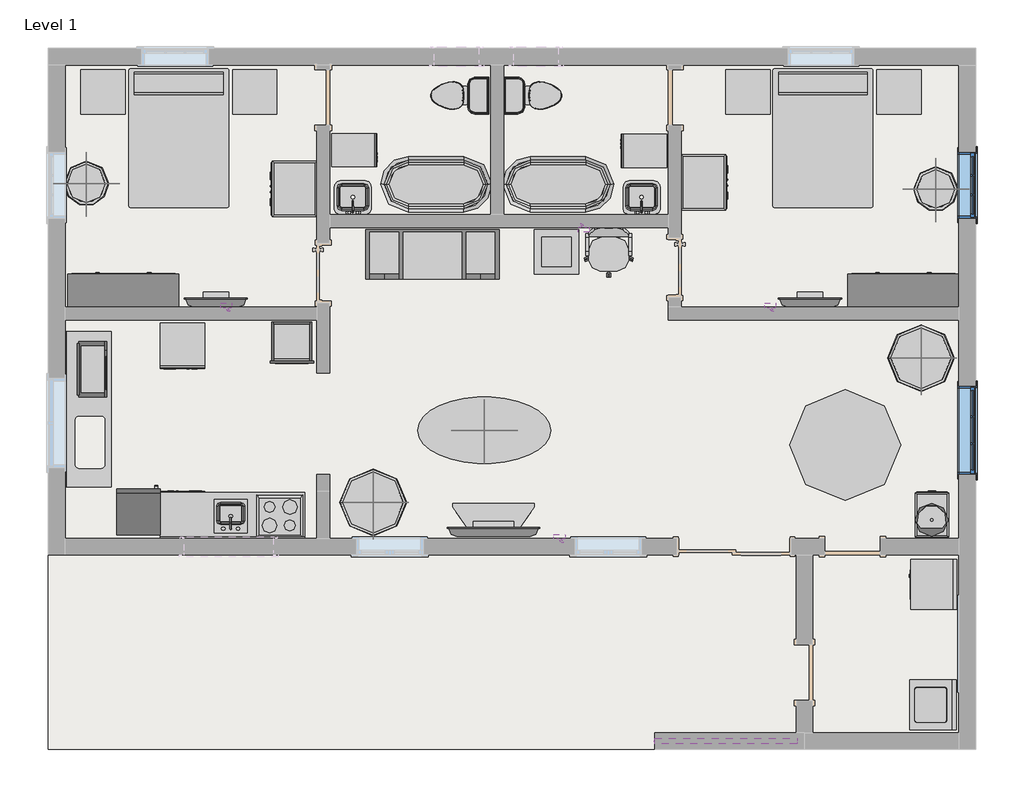
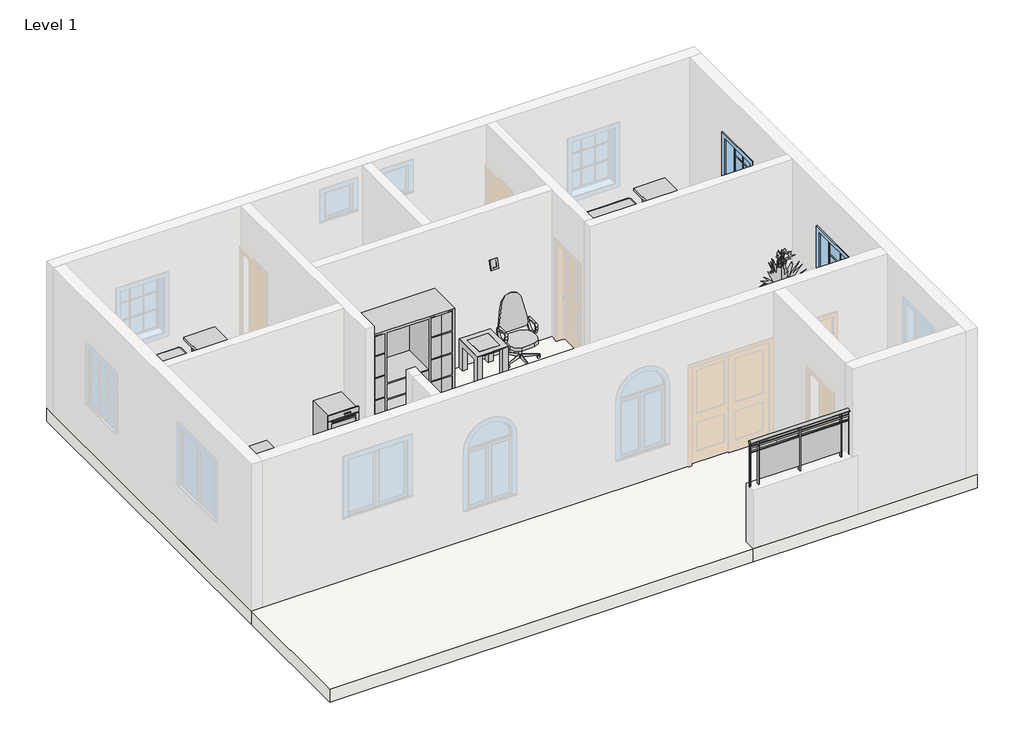
# One storey, part 2 of 2: 26 furniture elements, 15 proxies, 11 flow terminals, 5 geographic elements, 2 windows, 1 railing, 1 slab.
"""IFC4 building model written with IfcOpenShell, lengths in millimetres."""

from ifc_helpers import new_model, si_unit, point, frame, origin, place, context, project, spatial, polyline, ellipse_curve, trimmed, outline, extrude, transform, mapped, element, save
from ifc_brep_helpers import plane_surface, extruded_surface, advanced_brep
from components import proxy_7e1014cc, proxy_a6faaae8, proxy_45b28599, proxy_b4d0e45e, kitchenette_medium_kitchenette_medium_844211aa, proxy_8a8d5ab2, proxy_8b8c2dc4, rpc_picture_frame_rpc_picture_frame_c25e3fe9, proxy_c523a7b7, proxy_718fa39f, flow_terminal_accce45a, flow_terminal_871c2e40, flow_terminal_d49f872f, flow_terminal_62a433f7, toilet_domestic_3d_toilet_domestic_3d_f7549cf7, toilet_domestic_3d_toilet_domestic_3d_183bbd19, flow_terminal_b374fae2, furniture_338da5bd, furniture_fb2da572, furniture_0253826f, chair_executive_chair_executive_8d69e98c, furniture_c6510c7c, furniture_ac03d711, furniture_06d35bcb, furniture_cf0b6580, furniture_56245f3a, furniture_fdf74506, tv_stand_tv_stand_6ce107e5, furniture_b5c51a22, furniture_bbcc68ce, furniture_027a2ad9, furniture_5bc9ed15, table_round_2_c80d6d9c, furniture_a0cc3393, rpc_plant_tropical_55f6ff97, rpc_plant_tropical_agave_1_5_93a2a214, window_642cfea4, window_544f1267

model = new_model("IFC4")

# Units and contexts
model_context = context("Model", 3, world=origin())
ifc_project = project(units=[si_unit("LENGTHUNIT", "METRE", prefix="MILLI")], contexts=[model_context])

# Site, building, storey
site = spatial("IfcSite", under=ifc_project)
building = spatial("IfcBuilding", under=site)
storey = spatial("IfcBuildingStorey", under=building, Name="Level 1", Elevation=0.0)

# Proxies
placement = place(None, origin())
proxy_shape = proxy_7e1014cc(model_context)
element("IfcBuildingElementProxy", 1, Name="18\" x 24\" x 34 1/2\"", ObjectType="18\" x 24\" x 34 1/2\"", at=placement, inside=storey, context=model_context, shape_type="MappedRepresentation", body=[
    mapped(proxy_shape, transform((-2868.9943199, 12467.072386, 0.0), x_axis=(0.0, -1.0000000000000004, 0.0), y_axis=(1.0000000000000004, 0.0, 0.0), z_axis=(0.0, 0.0, 1.0))),
])
element("IfcBuildingElementProxy", 2, Name="18\" x 24\" x 34 1/2\"", ObjectType="18\" x 24\" x 34 1/2\"", at=placement, inside=storey, context=model_context, shape_type="MappedRepresentation", body=[
    mapped(proxy_shape, transform((-6323.8951903, 11867.537449, 0.0), x_axis=(0.0, 1.0, 0.0), y_axis=(-1.0, 0.0, 0.0), z_axis=(0.0, 0.0, 1.0))),
])
proxy_2_shape = proxy_a6faaae8(model_context)
element("IfcBuildingElementProxy", 3, Name="Cook Top-4 Unit2 : 22\" x 20\"", ObjectType="Cook Top-4 Unit2 : 22\" x 20\"", at=placement, inside=storey, context=model_context, shape_type="MappedRepresentation", body=[
    mapped(proxy_2_shape, transform((-7606.3447551, 7144.4549175, 0.0), x_axis=(-1.0000000000000004, 0.0, 0.0), y_axis=(0.0, -1.0000000000000004, 0.0), z_axis=(0.0, 0.0, 1.0))),
])
proxy_3_shape = proxy_45b28599(model_context)
element("IfcBuildingElementProxy", 4, Name="Dishwasher : 24\" x 24\" x 34\"", ObjectType="Dishwasher : 24\" x 24\" x 34\"", at=placement, inside=storey, context=model_context, shape_type="MappedRepresentation", body=[
    mapped(proxy_3_shape, transform((-8557.5272866, 7436.3044823, 0.0), x_axis=(-1.0000000000000004, 0.0, 0.0), y_axis=(0.0, -1.0000000000000004, 0.0), z_axis=(0.0, 0.0, 1.0))),
])
element("IfcBuildingElementProxy", 5, Name="Dishwasher : 24\" x 24\" x 34\"", ObjectType="Dishwasher : 24\" x 24\" x 34\"", at=placement, inside=storey, context=model_context, shape_type="MappedRepresentation", body=[
    mapped(proxy_3_shape, transform((-9322.1622236, 9227.5053528, 0.0), x_axis=(1.0, 0.0, 0.0), y_axis=(0.0, 1.0, 0.0), z_axis=(0.0, 0.0, 1.0))),
])
proxy_4_shape = proxy_b4d0e45e(model_context)
element("IfcBuildingElementProxy", 6, Name="Dryer : 27\" x 25\" x 35\"", ObjectType="Dryer : 27\" x 25\" x 35\"", at=placement, inside=storey, context=model_context, shape_type="MappedRepresentation", body=[
    mapped(proxy_4_shape, transform((1055.0552449, 6585.6549175, 0.0), x_axis=(0.0, -1.0000000000000004, 0.0), y_axis=(1.0000000000000004, 0.0, 0.0), z_axis=(0.0, 0.0, 1.0))),
])
kitchenette_medium_kitchenette_medium_shape = kitchenette_medium_kitchenette_medium_844211aa(model_context)
element("IfcBuildingElementProxy", 7, Name="Kitchenette - Medium : Kitchenette - Medium", ObjectType="Kitchenette - Medium : Kitchenette - Medium", at=placement, inside=storey, context=model_context, shape_type="MappedRepresentation", body=[
    mapped(kitchenette_medium_kitchenette_medium_shape, transform((-7930.5070502, 6839.6549175, 0.0), x_axis=(-1.0000000000000004, 0.0, 0.0), y_axis=(0.0, -1.0000000000000004, 0.0), z_axis=(0.0, 0.0, 1.0))),
])
proxy_5_shape = proxy_8a8d5ab2(model_context)
element("IfcBuildingElementProxy", 8, Name="Microwave : 30\" x 16\" x 18\"", ObjectType="Microwave : 30\" x 16\" x 18\"", at=placement, inside=storey, context=model_context, shape_type="MappedRepresentation", body=[
    mapped(proxy_5_shape, transform((-10537.525261, 8663.4620402, 0.0), x_axis=(0.0, 1.0, 0.0), y_axis=(-1.0, 0.0, 0.0), z_axis=(0.0, 0.0, 1.0))),
])
proxy_6_shape = proxy_8b8c2dc4(model_context)
element("IfcBuildingElementProxy", 9, Name="Oven Double-Built-in : 21 1/2\" x 39 1/4\" x 21\"", ObjectType="Oven Double-Built-in : 21 1/2\" x 39 1/4\" x 21\"", at=placement, inside=storey, context=model_context, shape_type="MappedRepresentation", body=[
    mapped(proxy_6_shape, transform((-7406.0698278, 9403.6890586, 0.0), x_axis=(1.0, 0.0, 0.0), y_axis=(0.0, 1.0, 0.0), z_axis=(0.0, 0.0, 1.0))),
])
rpc_picture_frame_rpc_picture_frame_shape = rpc_picture_frame_rpc_picture_frame_c25e3fe9(model_context)
element("IfcBuildingElementProxy", 10, Name="RPC Picture Frame : RPC Picture Frame", ObjectType="RPC Picture Frame : RPC Picture Frame", at=placement, inside=storey, context=model_context, shape_type="MappedRepresentation", body=[
    mapped(rpc_picture_frame_rpc_picture_frame_shape, transform((-8339.9401773, 10014.6549175, 1828.8), x_axis=(-1.0000000000000004, 0.0, 0.0), y_axis=(0.0, -1.0000000000000004, 0.0), z_axis=(0.0, 0.0, 1.0))),
])
element("IfcBuildingElementProxy", 11, Name="RPC Picture Frame : RPC Picture Frame", ObjectType="RPC Picture Frame : RPC Picture Frame", at=placement, inside=storey, context=model_context, shape_type="MappedRepresentation", body=[
    mapped(rpc_picture_frame_rpc_picture_frame_shape, transform((-876.145624, 10014.6549175, 1828.8), x_axis=(-1.0, 0.0, 0.0), y_axis=(0.0, -1.0, 0.0), z_axis=(0.0, 0.0, 1.0))),
])
element("IfcBuildingElementProxy", 12, Name="RPC Picture Frame : RPC Picture Frame", ObjectType="RPC Picture Frame : RPC Picture Frame", at=placement, inside=storey, context=model_context, shape_type="MappedRepresentation", body=[
    mapped(rpc_picture_frame_rpc_picture_frame_shape, transform((-3766.7525994, 6839.6549175, 1828.8), x_axis=(-1.0000000000000004, 0.0, 0.0), y_axis=(0.0, -1.0000000000000004, 0.0), z_axis=(0.0, 0.0, 1.0))),
])
element("IfcBuildingElementProxy", 13, Name="RPC Picture Frame : RPC Picture Frame", ObjectType="RPC Picture Frame : RPC Picture Frame", at=placement, inside=storey, context=model_context, shape_type="MappedRepresentation", body=[
    mapped(rpc_picture_frame_rpc_picture_frame_shape, transform((-3433.7801384, 11106.8549175, 1828.8), x_axis=(1.0, 0.0, 0.0), y_axis=(0.0, 1.0, 0.0), z_axis=(0.0, 0.0, 1.0))),
])
proxy_7_shape = proxy_c523a7b7(model_context)
element("IfcBuildingElementProxy", 14, Name="Refrigerator : 24\" x 25\" LH", ObjectType="Refrigerator : 24\" x 25\" LH", at=placement, inside=storey, context=model_context, shape_type="MappedRepresentation", body=[
    mapped(proxy_7_shape, transform((-9543.0947551, 7190.103889, 0.0), x_axis=(-1.0000000000000004, 0.0, 0.0), y_axis=(0.0, -1.0000000000000004, 0.0), z_axis=(0.0, 0.0, 1.0))),
])
proxy_8_shape = proxy_718fa39f(model_context)
element("IfcBuildingElementProxy", 15, Name="Washer : 27\" x 25\" x 35\"", ObjectType="Washer : 27\" x 25\" x 35\"", at=placement, inside=storey, context=model_context, shape_type="MappedRepresentation", body=[
    mapped(proxy_8_shape, transform((1080.7056801, 4974.072386, 0.0), x_axis=(0.0, -1.0, 0.0), y_axis=(1.0, 0.0, 0.0), z_axis=(0.0, 0.0, 1.0))),
])

# Flow terminals
flow_terminal_shape = flow_terminal_accce45a(model_context)
element("IfcFlowTerminal", 16, ObjectType="Floor Drain - Round : 5\" Strainer - 2\" Drain", at=placement, inside=storey, context=model_context, shape_type="MappedRepresentation", body=[
    mapped(flow_terminal_shape, transform((-4291.6447551, 12313.3549175, 0.0), x_axis=(1.0, 0.0, 0.0), y_axis=(0.0, 1.0, 0.0), z_axis=(0.0, 0.0, 1.0))),
])
element("IfcFlowTerminal", 17, ObjectType="Floor Drain - Round : 5\" Strainer - 2\" Drain", at=placement, inside=storey, context=model_context, shape_type="MappedRepresentation", body=[
    mapped(flow_terminal_shape, transform((-4952.0447551, 12338.7549175, 0.0), x_axis=(1.0, 0.0, 0.0), y_axis=(0.0, 1.0, 0.0), z_axis=(0.0, 0.0, 1.0))),
])
element("IfcFlowTerminal", 18, ObjectType="Floor Drain - Round : 5\" Strainer - 2\" Drain", at=placement, inside=storey, context=model_context, shape_type="MappedRepresentation", body=[
    mapped(flow_terminal_shape, transform((788.3552449, 4337.7549175, 0.0), x_axis=(0.0, 1.0, 0.0), y_axis=(-1.0, 0.0, 0.0), z_axis=(0.0, 0.0, 1.0))),
])
flow_terminal_2_shape = flow_terminal_871c2e40(model_context)
element("IfcFlowTerminal", 19, ObjectType="Sink Kitchen-Island : 18\" x 18\"", at=placement, inside=storey, context=model_context, shape_type="MappedRepresentation", body=[
    mapped(flow_terminal_2_shape, transform((-8263.7555146, 7146.8003187, -14.4), x_axis=(-1.0000000000000004, 0.0, 0.0), y_axis=(0.0, -1.0000000000000004, 0.0), z_axis=(0.0, 0.0, 1.0))),
])
flow_terminal_3_shape = flow_terminal_d49f872f(model_context)
element("IfcFlowTerminal", 20, ObjectType="Sink Vanity-Round : 19\" x 19\"", at=placement, inside=storey, context=model_context, shape_type="MappedRepresentation", body=[
    mapped(flow_terminal_3_shape, transform((1437.4569854, 7180.500516, 431.8), x_axis=(-1.0000000000000004, 0.0, 0.0), y_axis=(0.0, -1.0000000000000004, 0.0), z_axis=(0.0, 0.0, 1.0))),
])
flow_terminal_4_shape = flow_terminal_62a433f7(model_context)
element("IfcFlowTerminal", 21, ObjectType="Sink Vanity-Square : 20\" x 18\"", at=placement, inside=storey, context=model_context, shape_type="MappedRepresentation", body=[
    mapped(flow_terminal_4_shape, transform((-6587.3555146, 11477.5003187, 0.0), x_axis=(-1.0000000000000004, 0.0, 0.0), y_axis=(0.0, -1.0000000000000004, 0.0), z_axis=(0.0, 0.0, 1.0))),
])
element("IfcFlowTerminal", 22, ObjectType="Sink Vanity-Square : 20\" x 18\"", at=placement, inside=storey, context=model_context, shape_type="MappedRepresentation", body=[
    mapped(flow_terminal_4_shape, transform((-2624.9555146, 11477.5003187, 0.0), x_axis=(-1.0, 0.0, 0.0), y_axis=(0.0, -1.0, 0.0), z_axis=(0.0, 0.0, 1.0))),
])
toilet_domestic_3d_toilet_domestic_3d_shape = toilet_domestic_3d_toilet_domestic_3d_f7549cf7(model_context)
toilet_domestic_3d_toilet_domestic_3d_2_shape = toilet_domestic_3d_toilet_domestic_3d_183bbd19(model_context)
element("IfcFlowTerminal", 23, ObjectType="Toilet-Domestic-3D : Toilet-Domestic-3D", at=placement, inside=storey, context=model_context, shape_type="MappedRepresentation", body=[
    mapped(toilet_domestic_3d_toilet_domestic_3d_shape, transform((-5230.8407825, 12922.9549175, 0.0), x_axis=(0.0, -1.0000000000000004, 0.0), y_axis=(1.0000000000000004, 0.0, 0.0), z_axis=(0.0, 0.0, 1.0))),
    mapped(toilet_domestic_3d_toilet_domestic_3d_2_shape, transform((-5230.8407825, 12922.9549175, 0.0), x_axis=(0.0, -1.0000000000000004, 0.0), y_axis=(1.0000000000000004, 0.0, 0.0), z_axis=(0.0, 0.0, 1.0))),
])
element("IfcFlowTerminal", 24, ObjectType="Toilet-Domestic-3D : Toilet-Domestic-3D", at=placement, inside=storey, context=model_context, shape_type="MappedRepresentation", body=[
    mapped(toilet_domestic_3d_toilet_domestic_3d_shape, transform((-4038.2487278, 12922.9549175, 0.0), x_axis=(0.0, 1.0000000000000004, 0.0), y_axis=(-1.0000000000000004, 0.0, 0.0), z_axis=(0.0, 0.0, 1.0))),
    mapped(toilet_domestic_3d_toilet_domestic_3d_2_shape, transform((-4038.2487278, 12922.9549175, 0.0), x_axis=(0.0, 1.0000000000000004, 0.0), y_axis=(-1.0000000000000004, 0.0, 0.0), z_axis=(0.0, 0.0, 1.0))),
])
flow_terminal_5_shape = flow_terminal_b374fae2(model_context)
element("IfcFlowTerminal", 25, ObjectType="Tub-Free Standing-3D : 30\" x 60\"", at=placement, inside=storey, context=model_context, shape_type="MappedRepresentation", body=[
    mapped(flow_terminal_5_shape, transform((-5460.0447551, 11703.7549175, 0.0), x_axis=(0.0, -1.0000000000000004, 0.0), y_axis=(1.0000000000000004, 0.0, 0.0), z_axis=(0.0, 0.0, 1.0))),
])
element("IfcFlowTerminal", 26, ObjectType="Tub-Free Standing-3D : 30\" x 60\"", at=placement, inside=storey, context=model_context, shape_type="MappedRepresentation", body=[
    mapped(flow_terminal_5_shape, transform((-3784.2487278, 11703.7549175, 0.0), x_axis=(0.0, 1.0000000000000002, 0.0), y_axis=(-1.0000000000000002, 0.0, 0.0), z_axis=(0.0, 0.0, 1.0))),
])

# Furniture
furniture_shape = furniture_338da5bd(model_context)
element("IfcFurniture", 27, ObjectType="30\"", at=placement, inside=storey, context=model_context, shape_type="MappedRepresentation", body=[
    mapped(furniture_shape, transform((-2094.5447551, 11710.4172126, 0.0), x_axis=(0.0, 1.0000000000000002, 0.0), y_axis=(-1.0000000000000002, 0.0, 0.0), z_axis=(0.0, 0.0, 1.0))),
])
element("IfcFurniture", 28, ObjectType="30\"", at=placement, inside=storey, context=model_context, shape_type="MappedRepresentation", body=[
    mapped(furniture_shape, transform((-7098.3447551, 11658.9926225, 0.0), x_axis=(0.0, -1.0000000000000002, 0.0), y_axis=(1.0000000000000002, 0.0, 0.0), z_axis=(0.0, 0.0, 1.0))),
])
furniture_2_shape = furniture_fb2da572(model_context)
element("IfcFurniture", 29, ObjectType="Base Cabinet-4 Drawers : 18\"", at=placement, inside=storey, context=model_context, shape_type="MappedRepresentation", body=[
    mapped(furniture_2_shape, transform((1365.8929498, 6858.7049175, 0.0), x_axis=(-1.0, 0.0, 0.0), y_axis=(0.0, -1.0, 0.0), z_axis=(0.0, 0.0, 1.0))),
])
furniture_3_shape = furniture_0253826f(model_context)
element("IfcFurniture", 30, ObjectType="Bed-Standard.0001 : Double 54\" x 75\"", at=placement, inside=storey, context=model_context, shape_type="MappedRepresentation", body=[
    mapped(furniture_3_shape, transform((-9262.1332797, 12384.3499995, 0.0), x_axis=(1.0, 0.0, 0.0), y_axis=(0.0, 1.0, 0.0), z_axis=(0.0, 0.0, 1.0))),
])
element("IfcFurniture", 31, ObjectType="Bed-Standard.0001 : Double 54\" x 75\"", at=placement, inside=storey, context=model_context, shape_type="MappedRepresentation", body=[
    mapped(furniture_3_shape, transform((-422.9332797, 12384.3499995, 0.0), x_axis=(1.0, 0.0, 0.0), y_axis=(0.0, 1.0, 0.0), z_axis=(0.0, 0.0, 1.0))),
])
chair_executive_chair_executive_shape = chair_executive_chair_executive_8d69e98c(model_context)
element("IfcFurniture", 32, ObjectType="Chair-Executive : Chair-Executive", at=placement, inside=storey, context=model_context, shape_type="MappedRepresentation", body=[
    mapped(chair_executive_chair_executive_shape, transform((-2950.5039355, 10795.6008192, 0.0), x_axis=(-1.0000000000000004, 0.0, 0.0), y_axis=(0.0, -1.0000000000000004, 0.0), z_axis=(0.0, 0.0, 1.0))),
])
furniture_4_shape = furniture_c6510c7c(model_context)
element("IfcFurniture", 33, ObjectType="Counter Top w Sink Hole : 24\" Depth", at=placement, inside=storey, context=model_context, shape_type="MappedRepresentation", body=[
    mapped(furniture_4_shape, transform((-8463.9070502, 6839.6549175, -14.4), x_axis=(-1.0000000000000004, 0.0, 0.0), y_axis=(0.0, -1.0000000000000004, 0.0), z_axis=(0.0, 0.0, 1.0))),
])
furniture_5_shape = furniture_ac03d711(model_context)
element("IfcFurniture", 34, ObjectType="Counter Top w Sink Hole : 24\" Depth", at=placement, inside=storey, context=model_context, shape_type="MappedRepresentation", body=[
    mapped(furniture_5_shape, transform((-10552.7447551, 8751.3172126, 0.0), x_axis=(0.0, 1.0000000000000002, 0.0), y_axis=(-1.0000000000000002, 0.0, 0.0), z_axis=(0.0, 0.0, 1.0))),
])
furniture_6_shape = furniture_06d35bcb(model_context)
element("IfcFurniture", 35, ObjectType="Dresser : 72\" x 60\" x 18\"", at=placement, inside=storey, context=model_context, shape_type="MappedRepresentation", body=[
    mapped(furniture_6_shape, transform((-10021.838015, 9880.0919634, 0.0), x_axis=(-1.0000000000000004, 0.0, 0.0), y_axis=(0.0, -1.0000000000000004, 0.0), z_axis=(0.0, 0.0, 1.0))),
])
element("IfcFurniture", 36, ObjectType="Dresser : 72\" x 60\" x 18\"", at=placement, inside=storey, context=model_context, shape_type="MappedRepresentation", body=[
    mapped(furniture_6_shape, transform((684.261985, 9880.0919634, 0.0), x_axis=(-1.0000000000000004, 0.0, 0.0), y_axis=(0.0, -1.0000000000000004, 0.0), z_axis=(0.0, 0.0, 1.0))),
])
furniture_7_shape = furniture_cf0b6580(model_context)
element("IfcFurniture", 37, ObjectType="Entertainment Center : 72\" x 72\" x 24\"", at=placement, inside=storey, context=model_context, shape_type="MappedRepresentation", body=[
    mapped(furniture_7_shape, transform((-5510.8447551, 11183.0549175, 0.0), x_axis=(1.0, 0.0, 0.0), y_axis=(0.0, 1.0, 0.0), z_axis=(0.0, 0.0, 1.0))),
])
furniture_8_shape = furniture_56245f3a(model_context)
element("IfcFurniture", 38, ObjectType="TV - Flat Screen : 32\"", at=placement, inside=storey, context=model_context, shape_type="MappedRepresentation", body=[
    mapped(furniture_8_shape, transform((-333.1892693, 10073.1935412, 914.4), x_axis=(-1.0, 0.0, 0.0), y_axis=(0.0, -1.0, 0.0), z_axis=(0.0, 0.0, 1.0))),
])
element("IfcFurniture", 39, ObjectType="TV - Flat Screen : 32\"", at=placement, inside=storey, context=model_context, shape_type="MappedRepresentation", body=[
    mapped(furniture_8_shape, transform((-8486.5892693, 10073.1935412, 914.4), x_axis=(-1.0000000000000004, 0.0, 0.0), y_axis=(0.0, -1.0000000000000004, 0.0), z_axis=(0.0, 0.0, 1.0))),
])
furniture_9_shape = furniture_fdf74506(model_context)
element("IfcFurniture", 40, ObjectType="TV - Flat Screen : 50\"", at=placement, inside=storey, context=model_context, shape_type="MappedRepresentation", body=[
    mapped(furniture_9_shape, transform((-4676.5892693, 6923.5935412, 914.4), x_axis=(-1.0, 0.0, 0.0), y_axis=(0.0, -1.0, 0.0), z_axis=(0.0, 0.0, 1.0))),
])
tv_stand_tv_stand_shape = tv_stand_tv_stand_6ce107e5(model_context)
element("IfcFurniture", 41, ObjectType="TV Stand : TV Stand", at=placement, inside=storey, context=model_context, shape_type="MappedRepresentation", body=[
    mapped(tv_stand_tv_stand_shape, transform((-4547.4567531, 6865.0549175, 0.0), x_axis=(-1.0000000000000004, 0.0, 0.0), y_axis=(0.0, -1.0000000000000004, 0.0), z_axis=(0.0, 0.0, 1.0))),
])
furniture_10_shape = furniture_b5c51a22(model_context)
element("IfcFurniture", 42, ObjectType="Table-Coffee : 24\" x 24\" x 24\"", at=placement, inside=storey, context=model_context, shape_type="MappedRepresentation", body=[
    mapped(furniture_10_shape, transform((-3827.3105218, 10681.4438397, 0.0), x_axis=(1.0, 0.0, 0.0), y_axis=(0.0, 1.0, 0.0), z_axis=(0.0, 0.0, 1.0))),
])
furniture_11_shape = furniture_bbcc68ce(model_context)
element("IfcFurniture", 43, ObjectType="Table-Dining Round w Chairs : 60\" Diameter", at=placement, inside=storey, context=model_context, shape_type="MappedRepresentation", body=[
    mapped(furniture_11_shape, transform((49.6732777, 8307.2336061, 0.0), x_axis=(1.0, 0.0, 0.0), y_axis=(0.0, 1.0, 0.0), z_axis=(0.0, 0.0, 1.0))),
])
furniture_12_shape = furniture_027a2ad9(model_context)
element("IfcFurniture", 44, ObjectType="Table-Ellipse : 72\" x 36\"", at=placement, inside=storey, context=model_context, shape_type="MappedRepresentation", body=[
    mapped(furniture_12_shape, transform((-4799.6447551, 8325.5549175, 0.0), x_axis=(1.0, 0.0, 0.0), y_axis=(0.0, 1.0, 0.0), z_axis=(0.0, 0.0, 1.0))),
])
furniture_13_shape = furniture_5bc9ed15(model_context)
element("IfcFurniture", 45, ObjectType="Table-Night Stand : 24\" x 24\" x 30\"", at=placement, inside=storey, context=model_context, shape_type="MappedRepresentation", body=[
    mapped(furniture_13_shape, transform((-10340.5783854, 12668.9549175, 0.0), x_axis=(1.0, 0.0, 0.0), y_axis=(0.0, 1.0, 0.0), z_axis=(0.0, 0.0, 1.0))),
])
element("IfcFurniture", 46, ObjectType="Table-Night Stand : 24\" x 24\" x 30\"", at=placement, inside=storey, context=model_context, shape_type="MappedRepresentation", body=[
    mapped(furniture_13_shape, transform((-8257.7783854, 12668.9549175, 0.0), x_axis=(1.0, 0.0, 0.0), y_axis=(0.0, 1.0, 0.0), z_axis=(0.0, 0.0, 1.0))),
])
element("IfcFurniture", 47, ObjectType="Table-Night Stand : 24\" x 24\" x 30\"", at=placement, inside=storey, context=model_context, shape_type="MappedRepresentation", body=[
    mapped(furniture_13_shape, transform((-1488.6783854, 12668.9549175, 0.0), x_axis=(1.0, 0.0, 0.0), y_axis=(0.0, 1.0, 0.0), z_axis=(0.0, 0.0, 1.0))),
])
element("IfcFurniture", 48, ObjectType="Table-Night Stand : 24\" x 24\" x 30\"", at=placement, inside=storey, context=model_context, shape_type="MappedRepresentation", body=[
    mapped(furniture_13_shape, transform((581.4216146, 12668.9549175, 0.0), x_axis=(1.0, 0.0, 0.0), y_axis=(0.0, 1.0, 0.0), z_axis=(0.0, 0.0, 1.0))),
])
table_round_2_shape = table_round_2_c80d6d9c(model_context)
element("IfcFurniture", 49, ObjectType="Table-Round : 2", at=placement, inside=storey, context=model_context, shape_type="MappedRepresentation", body=[
    mapped(table_round_2_shape, transform((1194.7552449, 9316.1549175, 0.0), x_axis=(1.0, 0.0, 0.0), y_axis=(0.0, 1.0, 0.0), z_axis=(0.0, 0.0, 1.0))),
])
element("IfcFurniture", 50, ObjectType="Table-Round : 2", at=placement, inside=storey, context=model_context, shape_type="MappedRepresentation", body=[
    mapped(table_round_2_shape, transform((-6323.6447551, 7334.9549175, 0.0), x_axis=(1.0, 0.0, 0.0), y_axis=(0.0, 1.0, 0.0), z_axis=(0.0, 0.0, 1.0))),
])
furniture_14_shape = furniture_a0cc3393(model_context)
element("IfcFurniture", 51, ObjectType="Table-Round : 36\" Diameter", at=placement, inside=storey, context=model_context, shape_type="MappedRepresentation", body=[
    mapped(furniture_14_shape, transform((1397.9552449, 11640.2549175, 0.0), x_axis=(1.0, 0.0, 0.0), y_axis=(0.0, 1.0, 0.0), z_axis=(0.0, 0.0, 1.0))),
])
element("IfcFurniture", 52, ObjectType="Table-Round : 36\" Diameter", at=placement, inside=storey, context=model_context, shape_type="MappedRepresentation", body=[
    mapped(furniture_14_shape, transform((-10260.6447551, 11716.4549175, 0.0), x_axis=(1.0, 0.0, 0.0), y_axis=(0.0, 1.0, 0.0), z_axis=(0.0, 0.0, 1.0))),
])

# Geographic elements
rpc_plant_tropical_shape = rpc_plant_tropical_55f6ff97(model_context)
element("IfcGeographicElement", 53, ObjectType="RPC Plant - Tropical", at=placement, inside=storey, context=model_context, shape_type="MappedRepresentation", body=[
    mapped(rpc_plant_tropical_shape, transform((-6323.6447551, 7334.9549175, 762.0), x_axis=(1.0, 0.0, 0.0), y_axis=(0.0, 1.0, 0.0), z_axis=(0.0, 0.0, 1.0))),
])
element("IfcGeographicElement", 54, ObjectType="RPC Plant - Tropical", at=placement, inside=storey, context=model_context, shape_type="MappedRepresentation", body=[
    mapped(rpc_plant_tropical_shape, transform((1194.7552449, 9316.1549175, 762.0), x_axis=(1.0, 0.0, 0.0), y_axis=(0.0, 1.0, 0.0), z_axis=(0.0, 0.0, 1.0))),
])
rpc_plant_tropical_agave_1_5_shape = rpc_plant_tropical_agave_1_5_93a2a214(model_context)
element("IfcGeographicElement", 55, ObjectType="RPC Plant - Tropical : Agave - 1.5'", at=placement, inside=storey, context=model_context, shape_type="MappedRepresentation", body=[
    mapped(rpc_plant_tropical_agave_1_5_shape, transform((-4799.6447551, 8325.5549175, 762.0), x_axis=(1.0, 0.0, 0.0), y_axis=(0.0, 1.0, 0.0), z_axis=(0.0, 0.0, 1.0))),
])
element("IfcGeographicElement", 56, ObjectType="RPC Plant - Tropical : Agave - 1.5'", at=placement, inside=storey, context=model_context, shape_type="MappedRepresentation", body=[
    mapped(rpc_plant_tropical_agave_1_5_shape, transform((-10260.6447551, 11716.4549175, 762.0), x_axis=(1.0, 0.0, 0.0), y_axis=(0.0, 1.0, 0.0), z_axis=(0.0, 0.0, 1.0))),
])
element("IfcGeographicElement", 57, ObjectType="RPC Plant - Tropical : Agave - 1.5'", at=placement, inside=storey, context=model_context, shape_type="MappedRepresentation", body=[
    mapped(rpc_plant_tropical_agave_1_5_shape, transform((1397.9552449, 11640.2549175, 762.0), x_axis=(1.0, 0.0, 0.0), y_axis=(0.0, 1.0, 0.0), z_axis=(0.0, 0.0, 1.0))),
])

# Railing
element("IfcRailing", 58, ObjectType="Glass Panel - Bottom Fill", at=placement, inside=storey, context=model_context, shape_type="SolidModel", body=[
    advanced_brep(
    [(-507.0447551, 4020.2549175, 2133.6), (-507.0447551, 4096.4549175, 2133.6), (-2462.8447551, 4020.2549175, 2133.6), (-2462.8447551, 4096.4549175, 2133.6)],
    [
        (0, 1, ellipse_curve(frame((-507.0447551, 4058.3549175, 2133.6), z_axis=(1.0, 0.0, 0.0), x_axis=(0.0, 1.0, 0.0)), 38.1, 28.575)),
        (1, 0, ellipse_curve(frame((-507.0447551, 4058.3549175, 2133.6), z_axis=(1.0, 0.0, 0.0), x_axis=(0.0, 1.0, 0.0)), 38.1, 28.575)),
        (2, 3, ellipse_curve(frame((-2462.8447551, 4058.3549175, 2133.6), z_axis=(-1.0, 0.0, 0.0), x_axis=(0.0, 1.0, 0.0)), 38.1, 28.575)),
        (3, 2, ellipse_curve(frame((-2462.8447551, 4058.3549175, 2133.6), z_axis=(-1.0, 0.0, 0.0), x_axis=(0.0, 1.0, 0.0)), 38.1, 28.575)),
        (0, 2),
        (3, 1),
    ],
    [
        plane_surface(frame((-507.0447551, 4058.3549175, 2133.6), z_axis=(1.0, 0.0, 0.0), x_axis=(0.0, -1.0, 0.0))),
        plane_surface(frame((-2462.8447551, 4058.3549175, 2133.6), z_axis=(-1.0, 0.0, 0.0), x_axis=(0.0, -1.0, 0.0))),
        extruded_surface(trimmed(ellipse_curve(frame((-2462.8447551, 4058.3549175, 2133.6), z_axis=(1.0, 0.0, 0.0), x_axis=(0.0, 1.0, 0.0)), 38.1, 28.575), [point((-2462.8447551, 4020.2549175, 2133.6))], [point((-2462.8447551, 4096.4549175, 2133.6))], True, "CARTESIAN"), (1955.8, 0.0, 0.0), 1955.8),
        extruded_surface(trimmed(ellipse_curve(frame((-2462.8447551, 4058.3549175, 2133.6), z_axis=(1.0, 0.0, 0.0), x_axis=(0.0, 1.0, 0.0)), 38.1, 28.575), [point((-2462.8447551, 4096.4549175, 2133.6))], [point((-2462.8447551, 4020.2549175, 2133.6))], True, "CARTESIAN"), (1955.8, 0.0, 0.0), 1955.8),
    ],
    [
        (0, [[1, 2]]),
        (1, [[3, 4]]),
        (2, [[-1, 5, -4, 6]]),
        (3, [[-2, -6, -3, -5]]),
    ],
),
    extrude(outline(polyline([(-507.0447551, 4071.0549175), (-507.0447551, 4045.6549175), (-2462.8447551, 4045.6549175), (-2462.8447551, 4071.0549175), (-507.0447551, 4071.0549175)])), frame((0.0, 0.0, 2019.3), z_axis=(0.0, 0.0, 1.0), x_axis=(1.0, 0.0, 0.0)), (0.0, 0.0, 1.0), 25.4),
    extrude(outline(polyline([(-507.0447551, 4071.0549175), (-507.0447551, 4045.6549175), (-2462.8447551, 4045.6549175), (-2462.8447551, 4071.0549175), (-507.0447551, 4071.0549175)])), frame((0.0, 0.0, 1917.7), z_axis=(0.0, 0.0, 1.0), x_axis=(1.0, 0.0, 0.0)), (0.0, 0.0, 1.0), 25.4),
    extrude(outline(polyline([(-2291.3947551, 4083.7549175), (-2291.3947551, 4032.9549175), (-2304.0947551, 4032.9549175), (-2304.0947551, 4083.7549175), (-2291.3947551, 4083.7549175)])), frame((0.0, 0.0, 1219.2), z_axis=(0.0, 0.0, 1.0), x_axis=(1.0, 0.0, 0.0)), (0.0, 0.0, 1.0), 885.6788223),
    extrude(outline(polyline([(-1484.9447551, 4051.8197605), (-2297.7447551, 4051.8197605), (-2297.7447551, 4058.1697605), (-1484.9447551, 4058.1697605), (-1484.9447551, 4051.8197605)])), frame((0.0, 0.0, 1320.8), z_axis=(0.0, 0.0, 1.0), x_axis=(1.0, 0.0, 0.0)), (0.0, 0.0, 1.0), 596.9),
    extrude(outline(polyline([(-1478.5947551, 4083.7549175), (-1478.5947551, 4032.9549175), (-1491.2947551, 4032.9549175), (-1491.2947551, 4083.7549175), (-1478.5947551, 4083.7549175)])), frame((0.0, 0.0, 1219.2), z_axis=(0.0, 0.0, 1.0), x_axis=(1.0, 0.0, 0.0)), (0.0, 0.0, 1.0), 885.6788223),
    extrude(outline(polyline([(-672.1447551, 4051.8197605), (-1484.9447551, 4051.8197605), (-1484.9447551, 4058.1697605), (-672.1447551, 4058.1697605), (-672.1447551, 4051.8197605)])), frame((0.0, 0.0, 1320.8), z_axis=(0.0, 0.0, 1.0), x_axis=(1.0, 0.0, 0.0)), (0.0, 0.0, 1.0), 596.9),
    extrude(outline(polyline([(-665.7947551, 4083.7549175), (-665.7947551, 4032.9549175), (-678.4947551, 4032.9549175), (-678.4947551, 4083.7549175), (-665.7947551, 4083.7549175)])), frame((0.0, 0.0, 1219.2), z_axis=(0.0, 0.0, 1.0), x_axis=(1.0, 0.0, 0.0)), (0.0, 0.0, 1.0), 885.6788223),
    extrude(outline(polyline([(-2450.1447551, 4067.8799175), (-2450.1447551, 4048.8299175), (-2469.1947551, 4048.8299175), (-2469.1947551, 4067.8799175), (-2450.1447551, 4067.8799175)])), frame((0.0, 0.0, 1219.2), z_axis=(0.0, 0.0, 1.0), x_axis=(1.0, 0.0, 0.0)), (0.0, 0.0, 1.0), 885.6788223),
    extrude(outline(polyline([(-500.6947551, 4067.8799175), (-500.6947551, 4048.8299175), (-519.7447551, 4048.8299175), (-519.7447551, 4067.8799175), (-500.6947551, 4067.8799175)])), frame((0.0, 0.0, 1219.2), z_axis=(0.0, 0.0, 1.0), x_axis=(1.0, 0.0, 0.0)), (0.0, 0.0, 1.0), 885.6788223),
])

# Slab
element("IfcSlab", 59, ObjectType="Wood Joist 10\" - Ceramic Tile", at=placement, inside=storey, context=model_context, shape_type="SweptSolid", body=[
    extrude(outline(polyline([(1944.0552449, 13570.6549175), (1944.0552449, 3944.0549175), (-2462.8447551, 3944.0549175), (-10781.3447551, 3944.0549175), (-10781.3447551, 6611.0549175), (-10781.3447551, 13570.6549175), (1944.0552449, 13570.6549175)])), frame((0.0, 0.0, -273.05), z_axis=(0.0, 0.0, 1.0), x_axis=(1.0, 0.0, 0.0)), (0.0, 0.0, 1.0), 273.05),
])

# Windows
window_shape = window_642cfea4(model_context)
element("IfcWindow", 60, ObjectType="Casement 3x3 with Trim : 36\" x 48\"", at=placement, inside=storey, context=model_context, shape_type="MappedRepresentation", body=[
    mapped(window_shape, transform((1829.7552449, 11691.0549175, 304.8), x_axis=(0.0, -1.0, 0.0), y_axis=(1.0, 0.0, 0.0), z_axis=(0.0, 0.0, 1.0))),
])
window_2_shape = window_544f1267(model_context)
element("IfcWindow", 61, ObjectType="Casement 3x3 with Trim : 48\" x 60\"", at=placement, inside=storey, context=model_context, shape_type="MappedRepresentation", body=[
    mapped(window_2_shape, transform((1829.7552449, 8325.5549175, 304.8), x_axis=(0.0, -1.0, 0.0), y_axis=(1.0, 0.0, 0.0), z_axis=(0.0, 0.0, 1.0))),
])

save(model, "model.ifc")

# Revit data of these elements
# Type "18\" x 24\" x 34 1/2\""
#   Label = "T"
#   Assembly Code = "E1090400"
#   Depth = 2' - 0"
#   Height = 2' - 10 1/2"
#   Width = 1' - 6"
#   Panel Face Material = Plastic, Opaque Black
#   Trach Compact. Material = Steel, Paint Finish, Ivory, Matte
#   Default Elevation = 0
# Type "Cook Top-4 Unit2 : 22\" x 20\""
#   Depth = 1' - 8"
#   Width = 1' - 10"
#   Burner Material = Steel, Chrome Plated
#   Cooktop Material = Steel, Polished
#   Default Elevation = 0
#   Assembly Code = ""
# Type "Dishwasher : 24\" x 24\" x 34\""
#   Label = "DW"
#   Assembly Code = "E1090400"
#   Depth = 2' - 0"
#   Height = 2' - 10"
#   Width = 2' - 0"
#   Dishwasher Material = Steel, Paint Finish, Ivory, Glossy
#   Panel Face Material = Plastic, Opaque Black
#   Default Elevation = 0
# Type "Dryer : 27\" x 25\" x 35\""
#   Label = "D"
#   Assembly Code = "E1090400"
#   Depth = 2' - 1"
#   Height = 2' - 11"
#   Width = 2' - 3"
#   Dryer Material = Steel, Paint Finish, Ivory, Glossy
#   Default Elevation = 0
# Type "Kitchenette - Medium : Kitchenette - Medium"
#   Assembly Code = "E1090400"
#   Counter Length = 6' - 6"
#   Cabinet Width = 4' - 6"
#   Cabinet Height = 2' - 10 1/2"
#   Cabinet Depth = 2' - 0"
#   Toe Depth = 0' - 3"
#   Toe Height = 0' - 3 1/2"
#   Cabinet Material = Cabinets
#   Door/Drawer Material = Cabinets
#   Handle Material = Cabinets - Handles
#   Default Elevation = 0
# Type "Microwave : 30\" x 16\" x 18\""
#   Assembly Code = "E1090400"
#   Depth = 1' - 4"
#   Height = 1' - 6"
#   Width = 2' - 6"
#   Microwave Material = Laminate, Ivory, Matte
#   Default Elevation = 0
# Type "Oven Double-Built-in : 21 1/2\" x 39 1/4\" x 21\""
#   Label = "OVEN"
#   Assembly Code = "E1090400"
#   Depth = 1' - 9"
#   Height = 3' - 3 1/4"
#   Width = 1' - 9 1/2"
#   Oven Material = Metal - Stainless Steel, Polished
#   Default Elevation = 0
# Type "RPC Picture Frame : RPC Picture Frame"
#   built-in parameter 1005198 = "{2, 15},{39, RPC-16-8M5E-0H3T-F0AH-3U0K-JLQ7-G28B-AU},{1, 0},{1, 0},{2, 19},{1, 8},{5, Color},{1, 0},{1, 0},{3, 0.8},{3, 0.8},{3, 0.8},{1, 8},{7, BBoxMin},{1, 0},{1, 0},{1, 0},{1, 0},{1, 0},{1, 8},{7, BBoxMax},{1, 0},{1, 0},{1, 0},{1, 0},{1, 0},{2, 11},{9, RPCTypeId},{1, 0},{1, 0},{39, RPC-16-8M5E-0H3T-F0AH-3U0K-JLQ7-G28B-AU},{1, 6},{14, RPCPlantHeight},{1, 0},{1, 0},{5, 0.625},{2, 11},{7, keyword},{1, 0},{1, 0},{33, :RPCs:Office Clutter:Geometry:RPC},{2, 11},{8, category},{1, 0},{1, 0},{14, Office Clutter},{2, 11},{12, LocalizedUID},{1, 0},{1, 0},{13, Picture Frame},{2, 14},{6, Height},{1, 0},{1, 0},{5, 0.625},{1, 2},{16, Cast Reflections},{1, 0},{1, 0},{1, 0},{1, 2},{8, Portrait},{1, 0},{1, 0},{1, 1},{1, 2},{5, Stand},{1, 0},{1, 0},{1, 1},{2, 11},{10, RPCL_Frame},{1, 0},{1, 0},{5, Frame},{1, 4},{14, Frame Material},{1, 0},{1, 0},{1, 0},{2, 11},{12, RPCL_Picture},{1, 0},{1, 0},{7, Picture},{2, 11},{15, Picture Preview},{1, 0},{1, 0},{65, __RPC:/object data/textures/object/Photo/Photo0/textures/Portrait},{2, 11},{17, i_Picture Preview},{1, 0},{1, 0},{0, },{1, 2},{18, Use Custom Picture},{1, 0},{1, 0},{1, 0},{2, 11},{17, Picture File Name},{1, 0},{1, 0},{0, },{21, assetlibrary_base.fbx},{1, 5},"
#   built-in parameter 1005195 = "RPC-16-8M5E-0H3T-F0AH-3U0K-JLQ7-G28B-AU"
#   Height = 0
# Type "Refrigerator : 24\" x 25\" LH"
#   Label = "REF."
#   Assembly Code = "E1090400"
#   Depth = 2' - 0 3/4"
#   Handle = 0' - 1 1/2"
#   Height = 5' - 3 1/2"
#   Rear Clearance = 0' - 2"
#   Top Door Height = 1' - 8"
#   Width = 1' - 11 1/2"
#   Material = Steel, Paint Finish, Ivory, Glossy
#   Default Elevation = 0
# Type "Washer : 27\" x 25\" x 35\""
#   Label = "W"
#   Assembly Code = "E1090400"
#   Depth = 2' - 1"
#   Height = 2' - 11"
#   Width = 2' - 3"
#   Washer Material = Steel, Paint Finish, Ivory, Matte
#   Default Elevation = 0
# Type "Floor Drain - Round : 5\" Strainer - 2\" Drain"
#   WFU = 2
#   Strainer Height = 0' - 3 1/4"
#   Strainer Radius = 0' - 2 1/2"
#   Strainer Diameter = 0' - 5"
#   Radius 6 = 0' - 0 5/8"
#   Radius 5 = 0' - 1 1/4"
#   Radius 4 = 0' - 1 7/8"
#   Radius 2 = 0' - 3.04167"
#   Radius 1 = 0' - 2.02083"
#   Radius 3 = 0' - 2 1/32"
#   Pipe Radius = 1"
#   Pipe Diameter = 2"
#   Height 2 = 0' - 0.725"
#   Height 1 = 0' - 1 13/16"
#   Body Radius = 0' - 4 1/16"
#   Body Height = 0' - 3 5/8"
#   Body Diameter = 0' - 8 1/8"
#   Drain Material = none
#   HWFU = 0
#   Default Elevation = 0
#   CWFU = 0
# Type "Sink Kitchen-Island : 18\" x 18\""
#   Assembly Code = "D2010410"
#   Counter Height = 3' - 0"
#   Depth = 1' - 6"
#   Width = 1' - 6"
#   Faucet Material = Steel, Polished
#   Sink Material = Steel, Polished
#   Default Elevation = 0
# Type "Sink Vanity-Round : 19\" x 19\""
#   Assembly Code = "D2010400"
#   Top Of Counter = 2' - 7"
#   Basin Material = Porcelain, Linen
#   Faucet Material = Steel, Polished
#   Default Elevation = 0
# Type "Sink Vanity-Square : 20\" x 18\""
#   Assembly Code = "D2010400"
#   Counter Height = 2' - 7"
#   Depth = 1' - 6"
#   Width = 1' - 8"
#   Basin Material = Porcelain, Linen
#   Faucet Material = Steel, Polished
#   Default Elevation = 0
# Type "Toilet-Domestic-3D : Toilet-Domestic-3D"
#   Assembly Code = "D2010110"
#   Toilet - Bowl/Basin Material = Porcelain, Linen
#   Toilet - Seat Material = Laminate, Linen, Matte
#   Default Elevation = 0
# Type "Tub-Free Standing-3D : 30\" x 60\""
#   Assembly Code = "D2010110"
#   Height = 1' - 6"
#   Length = 5' - 0"
#   Width = 2' - 6"
#   Tub Material = Porcelain, Ivory
#   Default Elevation = 0
# Type "30\""
#   Assembly Code = "C1030410"
#   Depth = 2' - 0"
#   Height = 2' - 10 1/2"
#   Toe Depth = 0' - 3"
#   Toe Height = 0' - 3 1/2"
#   Width = 2' - 6"
#   Cabinet Material = none
#   Door/Drawer Material = none
#   Handle Material = Cabinets - Handles
#   Default Elevation = 0
# Type "Base Cabinet-4 Drawers : 18\""
#   Assembly Code = "C1030410"
#   Depth = 2' - 0"
#   Height = 2' - 10 1/2"
#   Toe Depth = 0' - 3"
#   Toe Height = 0' - 3 1/2"
#   Width = 1' - 6"
#   Cabinet Material = none
#   Door/Drawer Material = none
#   Handle Material = Cabinets - Handles
#   Default Elevation = 0
# Type "Bed-Standard.0001 : Double 54\" x 75\""
#   Assembly Code = "E2020200"
#   Length = 6' - 3"
#   Width = 4' - 6"
#   Leg Material = Steel, Chrome Plated
#   Mattress Material = Plywood, Sheathing
#   Default Elevation = 0
# Type "Chair-Executive : Chair-Executive"
#   Assembly Code = "E2020200"
#   Base/Arms Material = Plastic, Opaque Black
#   Casters Material = Plastic, Opaque Black
#   Seat/Back Material = Textile - Slate Blue
#   Default Elevation = 0
# Type "Counter Top w Sink Hole : 24\" Depth"
#   Assembly Code = "C1030400"
#   Counter Thickness = 0' - 1 1/2"
#   Depth = 2' - 1"
#   Height = 3' - 0"
#   Length [instance default] = 8' - 0"
#   Sink Location [instance default] = 2' - 0"
#   Sink Location To Wall [instance default] = 0' - 6"
#   Sink Opening Depth [instance default] = 1' - 3"
#   Sink Opening Width [instance default] = 2' - 3"
#   Counter Top Material = none
#   Default Elevation = 0
# Type "Dresser : 72\" x 60\" x 18\""
#   Assembly Code = "E2020200"
#   Depth = 1' - 6"
#   Height = 5' - 0"
#   Width = 5' - 0"
#   Dresser Material = Laminate - Ivory, Glossy
#   Drawer Material = Laminate, Ivory, Matte
#   Knob Material = Cherry
#   Default Elevation = 0
# Type "Entertainment Center : 72\" x 72\" x 24\""
#   Assembly Code = "E2020200"
#   Center Width = 2' - 8"
#   Depth = 2' - 0"
#   Height = 6' - 0"
#   Width = 6' - 0"
#   Material = Wood - Teak
#   Default Elevation = 0
# Type "TV - Flat Screen : 32\""
#   SinAng = 0' - 0.0193"
#   L = 2' - 3.79372"
#   H = 1' - 3.6354"
#   Thickness = 0' - 4.33071"
#   Diagonal = 2' - 7.88976"
#   CosAng = 0' - 0.03431"
#   Stand [instance default] = yes
#   Default Elevation = 0
# Type "TV - Flat Screen : 50\""
#   SinAng = 0' - 0.0193"
#   L = 3' - 7.57782"
#   H = 2' - 0.51477"
#   Thickness = 0' - 4.33071"
#   Diagonal = 4' - 2"
#   CosAng = 0' - 0.03431"
#   Stand [instance default] = yes
#   Default Elevation = 0
# Type "TV Stand : TV Stand"
#   Depth = 1' - 6"
#   Width = 3' - 8"
#   Height = 1' - 7 1/2"
#   Finish = Melamine - Gray
#   Default Elevation = 0
# Type "Table-Coffee : 24\" x 24\" x 24\""
#   Assembly Code = "E2020200"
#   Height = 2' - 0"
#   Length = 2' - 0"
#   Width = 2' - 0"
#   Top Material = none
#   Frame Material = none
#   Default Elevation = 0
# Type "Table-Dining Round w Chairs : 60\" Diameter"
#   Assembly Code = "E2020200"
#   Radius = 2' - 6"
#   Diameter = 5' - 0"
#   Height = 2' - 6"
#   Chairs = 6
#   Base Material = Pine
#   Top Material = Laminate, Linen, Matte
#   Default Elevation = 0
# Type "Table-Ellipse : 72\" x 36\""
#   Assembly Code = "E2020200"
#   Half Width = 1' - 6"
#   Half Length = 3' - 0"
#   Height = 2' - 6"
#   Length = 6' - 0"
#   Width = 3' - 0"
#   Base Material = Birch
#   Top Material = Laminate - Black
#   Default Elevation = 0
# Type "Table-Night Stand : 24\" x 24\" x 30\""
#   Assembly Code = "E2020200"
#   Depth = 2' - 0"
#   Height = 2' - 6"
#   Width = 2' - 0"
#   Base Material = Birch
#   Top Material = Laminate, Ivory, Matte
#   Default Elevation = 0
# Type "Table-Round : 2"
#   Assembly Code = "E2020200"
#   Base Radius = 0' - 10"
#   Height = 2' - 6"
#   Radius = 1' - 6"
#   Base Material = Steel, Chrome Plated
#   Top Material = Birch
#   Default Elevation = 0
# Type "Table-Round : 36\" Diameter"
#   Assembly Code = "E2020200"
#   Base Radius = 0' - 10"
#   Height = 2' - 6"
#   Radius = 1' - 0"
#   Base Material = Steel, Chrome Plated
#   Top Material = Birch
#   Default Elevation = 0
# Type "RPC Plant - Tropical"
#   built-in parameter 1005198 = "{2, 15},{39, RPC-16-FWM5-GM7X-C67P-4000-ST1L-LVER-AU},{1, 0},{1, 0},{2, 13},{1, 8},{5, Color},{1, 0},{1, 0},{3, 0.8},{3, 0.8},{3, 0.8},{1, 8},{7, BBoxMin},{1, 0},{1, 0},{1, 0},{1, 0},{1, 0},{1, 8},{7, BBoxMax},{1, 0},{1, 0},{1, 0},{1, 0},{1, 0},{2, 11},{9, RPCTypeId},{1, 0},{1, 0},{39, RPC-16-FWM5-GM7X-C67P-4000-ST1L-LVER-AU},{1, 6},{14, RPCPlantHeight},{1, 0},{1, 0},{1, 3},{2, 11},{7, keyword},{1, 0},{1, 0},{35, :RPCs:Shrubs [General]:Geometry:RPC},{2, 11},{8, category},{1, 0},{1, 0},{16, Shrubs [General]},{2, 11},{12, LocalizedUID},{1, 0},{1, 0},{10, Crane Lily},{2, 14},{6, Height},{1, 0},{1, 0},{1, 3},{1, 2},{16, Cast Reflections},{1, 0},{1, 0},{1, 0},{1, 2},{12, Cast Shadows},{1, 0},{1, 0},{1, 1},{1, 2},{9, Lock View},{1, 0},{1, 0},{1, 0},{1, 4},{5, ViewC},{1, 0},{1, 0},{1, 0},{21, assetlibrary_base.fbx},{1, 5},"
#   built-in parameter 1005195 = "RPC-16-FWM5-GM7X-C67P-4000-ST1L-LVER-AU"
#   Assembly Code = "G2050500"
#   Height = 3' - 0"
#   Default Elevation = 0
# Type "RPC Plant - Tropical : Agave - 1.5'"
#   built-in parameter 1005198 = "{2, 15},{39, RPC-16-G1GJ-63FX-7K5P-N000-ST1L-LVER-AU},{1, 0},{1, 0},{2, 13},{1, 8},{5, Color},{1, 0},{1, 0},{3, 0.8},{3, 0.8},{3, 0.8},{1, 8},{7, BBoxMin},{1, 0},{1, 0},{1, 0},{1, 0},{1, 0},{1, 8},{7, BBoxMax},{1, 0},{1, 0},{1, 0},{1, 0},{1, 0},{2, 11},{9, RPCTypeId},{1, 0},{1, 0},{39, RPC-16-G1GJ-63FX-7K5P-N000-ST1L-LVER-AU},{1, 6},{14, RPCPlantHeight},{1, 0},{1, 0},{3, 1.5},{2, 11},{7, keyword},{1, 0},{1, 0},{35, :RPCs:Plants [General]:Geometry:RPC},{2, 11},{8, category},{1, 0},{1, 0},{16, Plants [General]},{2, 11},{12, LocalizedUID},{1, 0},{1, 0},{5, Agave},{2, 14},{6, Height},{1, 0},{1, 0},{3, 1.5},{1, 2},{16, Cast Reflections},{1, 0},{1, 0},{1, 0},{1, 2},{12, Cast Shadows},{1, 0},{1, 0},{1, 1},{1, 2},{9, Lock View},{1, 0},{1, 0},{1, 0},{1, 4},{5, ViewC},{1, 0},{1, 0},{1, 0},{21, assetlibrary_base.fbx},{1, 5},"
#   built-in parameter 1005195 = "RPC-16-G1GJ-63FX-7K5P-N000-ST1L-LVER-AU"
#   Type Comments = "Agave"
#   Assembly Code = "G2050500"
#   Height = 1' - 6"
#   Default Elevation = 0
# Type "Glass Panel - Bottom Fill"
#   Assembly Code = "C2010400"
#   built-in parameter 1008612 = 0.0416667 (stored number, unit not read)
#   built-in parameter 1008611 = 0.0416667 (stored number, unit not read)
#   built-in parameter 1008609 = 0.333333 (stored number, unit not read)
#   built-in parameter 1008604 = 0.166667 (stored number, unit not read)
#   built-in parameter 1008603 = 0.166667 (stored number, unit not read)
#   Railing Height = 3' - 0"
#   built-in parameter 1008630 = 2
#   built-in parameter 1008610 = 2
#   built-in parameter 1008618 = Baluster - Square : 3/4"
# Type "Wood Joist 10\" - Ceramic Tile"
#   Assembly Code = "B1010"
#   Function = 0
#   Layers, outside or top first: 0' - 0 1/4" "Tile, Mosaic, Gray" (function 5); 0' - 0 1/2" "Concrete, Cast-in-Place gray" (function 4); 0' - 0 3/4" "Plywood, Sheathing" (function 1); 0' - 9 1/4" "Structure, Wood Joist/Rafter Layer" (function 1)
# Type "Casement 3x3 with Trim : 36\" x 48\""
#   Type Mark = "11"
#   Construction Type Id = "GSP4R"
#   Assembly Code = "B2020100"
#   Analytic Construction = "1/8 in Pilkington single glazing"
#   Visual Light Transmittance = 0.9
#   Solar Heat Gain Coefficient = 0.78
#   Heat Transfer Coefficient (U) = 0.6496 BTU/(h·ft²·°F)
#   Height = 4' - 0"
#   Default Sill Height = 2' - 0"
#   Trim Projection - Ext. = 0' - 0 1/2"
#   Trim Projection - Int. = 0' - 0 3/4"
#   Trim Width - Exterior = 0' - 3 1/2"
#   Trim Width - Interior = 0' - 3 1/2"
#   Width = 3' - 0"
#   Window Inset = 0' - 0 3/4"
#   Define Thermal Properties by = 1
#   Glass Pane Material = Glass
#   Sash Material = Softwood, Lumber
#   Trim Exterior Material = Trim
#   Trim Interior Material = Trim
#   Wall Closure = (empty or 0)
# Type "Casement 3x3 with Trim : 48\" x 60\""
#   Type Mark = "12"
#   Construction Type Id = "GSP4R"
#   Assembly Code = "B2020100"
#   Analytic Construction = "1/8 in Pilkington single glazing"
#   Visual Light Transmittance = 0.9
#   Solar Heat Gain Coefficient = 0.78
#   Heat Transfer Coefficient (U) = 0.6496 BTU/(h·ft²·°F)
#   Height = 5' - 0"
#   Default Sill Height = 1' - 0"
#   Trim Projection - Ext. = 0' - 0 1/2"
#   Trim Projection - Int. = 0' - 0 3/4"
#   Trim Width - Exterior = 0' - 3 1/2"
#   Trim Width - Interior = 0' - 3 1/2"
#   Width = 4' - 0"
#   Window Inset = 0' - 0 3/4"
#   Define Thermal Properties by = 1
#   Glass Pane Material = Glass
#   Sash Material = Sash
#   Trim Exterior Material = Trim
#   Trim Interior Material = Trim
#   Wall Closure = (empty or 0)
# Elements 1, 2 (IfcBuildingElementProxy, "18\" x 24\" x 34 1/2\"")
#   Phase Created = New Construction
#   Materials on its faces: "Steel, Paint Finish, Ivory, Matte", "Plastic, Opaque Black"
# Element 3 (IfcBuildingElementProxy, "Cook Top-4 Unit2 : 22\" x 20\"")
#   Phase Created = New Construction
#   Materials on its faces: "Steel, Chrome Plated", "Steel, Polished"
# Elements 4, 5 (IfcBuildingElementProxy, "Dishwasher : 24\" x 24\" x 34\"")
#   Phase Created = New Construction
#   Materials on its faces: "Steel, Paint Finish, Ivory, Glossy", "Plastic, Opaque Black"
# Element 6 (IfcBuildingElementProxy, "Dryer : 27\" x 25\" x 35\"")
#   Phase Created = New Construction
#   Materials on its faces: "Steel, Paint Finish, Ivory, Glossy"
# Element 7 (IfcBuildingElementProxy, "Kitchenette - Medium : Kitchenette - Medium")
#   Phase Created = New Construction
#   Materials on its faces: "Cabinets", "Cabinets - Handles"
# Element 8 (IfcBuildingElementProxy, "Microwave : 30\" x 16\" x 18\"")
#   Phase Created = New Construction
#   Materials on its faces: "Laminate, Ivory, Matte", "Glass"
# Element 9 (IfcBuildingElementProxy, "Oven Double-Built-in : 21 1/2\" x 39 1/4\" x 21\"")
#   Phase Created = New Construction
#   Materials on its faces: "Steel", "Metal - Stainless Steel, Polished", "Glass"
# Elements 10, 11, 12, 13 (IfcBuildingElementProxy, "RPC Picture Frame : RPC Picture Frame")
#   Phase Created = New Construction
# Element 14 (IfcBuildingElementProxy, "Refrigerator : 24\" x 25\" LH")
#   Phase Created = New Construction
#   Materials on its faces: "Steel, Paint Finish, Ivory, Glossy", "Steel, Chrome Plated"
# Element 15 (IfcBuildingElementProxy, "Washer : 27\" x 25\" x 35\"")
#   Phase Created = New Construction
#   Materials on its faces: "Steel, Paint Finish, Ivory, Matte"
# Element 16 (IfcFlowTerminal, "Floor Drain - Round : 5\" Strainer - 2\" Drain")
#   Mark = "14"
#   Phase Created = New Construction
# Element 17 (IfcFlowTerminal, "Floor Drain - Round : 5\" Strainer - 2\" Drain")
#   Mark = "15"
#   Phase Created = New Construction
# Element 18 (IfcFlowTerminal, "Floor Drain - Round : 5\" Strainer - 2\" Drain")
#   Mark = "16"
#   Phase Created = New Construction
# Element 19 (IfcFlowTerminal, "Sink Kitchen-Island : 18\" x 18\"")
#   Mark = "10"
#   Phase Created = New Construction
#   Materials on its faces: "Steel, Polished"
# Element 20 (IfcFlowTerminal, "Sink Vanity-Round : 19\" x 19\"")
#   Mark = "13"
#   Phase Created = New Construction
#   Materials on its faces: "Porcelain, Linen", "Steel, Polished"
# Element 21 (IfcFlowTerminal, "Sink Vanity-Square : 20\" x 18\"")
#   Mark = "8"
#   Phase Created = New Construction
#   Materials on its faces: "Porcelain, Linen", "Steel, Polished"
# Element 22 (IfcFlowTerminal, "Sink Vanity-Square : 20\" x 18\"")
#   Mark = "9"
#   Phase Created = New Construction
#   Materials on its faces: "Porcelain, Linen", "Steel, Polished"
# Element 23 (IfcFlowTerminal, "Toilet-Domestic-3D : Toilet-Domestic-3D")
#   Mark = "1"
#   Phase Created = New Construction
#   Materials on its faces: "Porcelain, Linen", "Laminate, Linen, Matte"
# Element 24 (IfcFlowTerminal, "Toilet-Domestic-3D : Toilet-Domestic-3D")
#   Mark = "2"
#   Phase Created = New Construction
#   Materials on its faces: "Porcelain, Linen", "Laminate, Linen, Matte"
# Element 25 (IfcFlowTerminal, "Tub-Free Standing-3D : 30\" x 60\"")
#   Mark = "6"
#   Phase Created = New Construction
#   Materials on its faces: "Porcelain, Ivory"
# Element 26 (IfcFlowTerminal, "Tub-Free Standing-3D : 30\" x 60\"")
#   Mark = "7"
#   Phase Created = New Construction
#   Materials on its faces: "Porcelain, Ivory"
# Elements 27, 28 (IfcFurniture, "30\"")
#   Phase Created = New Construction
#   Materials on its faces: "Cabinets", "Cabinets - Handles"
# Element 29 (IfcFurniture, "Base Cabinet-4 Drawers : 18\"")
#   Phase Created = New Construction
#   Materials on its faces: "Cabinets", "Cabinets - Handles"
# Elements 30, 31 (IfcFurniture, "Bed-Standard.0001 : Double 54\" x 75\"")
#   Phase Created = New Construction
#   Materials on its faces: "Linen, White", "Steel, Chrome Plated"
# Element 32 (IfcFurniture, "Chair-Executive : Chair-Executive")
#   Phase Created = New Construction
#   Materials on its faces: "Plastic, Opaque Black", "Textile - Slate Blue"
# Element 33 (IfcFurniture, "Counter Top w Sink Hole : 24\" Depth")
#   Sink Opening Depth = 1' - 2"
#   Sink Location To Wall = 0' - 6"
#   Length = 6' - 6"
#   Sink Location = 3' - 4"
#   Sink Opening Width = 1' - 4"
#   Phase Created = New Construction
#   Materials on its faces: "Counter Top"
# Element 34 (IfcFurniture, "Counter Top w Sink Hole : 24\" Depth")
#   Sink Opening Width = 2' - 3"
#   Sink Opening Depth = 1' - 3"
#   Sink Location To Wall = 0' - 6"
#   Sink Location = 2' - 0"
#   Length = 7' - 0"
#   Phase Created = New Construction
#   Materials on its faces: "Counter Top"
# Elements 35, 36 (IfcFurniture, "Dresser : 72\" x 60\" x 18\"")
#   Phase Created = New Construction
#   Materials on its faces: "Laminate, Ivory, Matte", "Cherry", "Laminate - Ivory, Glossy"
# Element 37 (IfcFurniture, "Entertainment Center : 72\" x 72\" x 24\"")
#   Phase Created = New Construction
#   Materials on its faces: "Wood - Teak", "Steel, Chrome Plated", "Glass - Clear, Grey"
# Elements 38, 39 (IfcFurniture, "TV - Flat Screen : 32\"")
#   Stand = yes
#   Phase Created = New Construction
#   Materials on its faces: "TV - Black", "TV - Glass", "TV - Screen"
# Element 40 (IfcFurniture, "TV - Flat Screen : 50\"")
#   Stand = yes
#   Phase Created = New Construction
#   Materials on its faces: "TV - Black", "TV - Glass", "TV - Screen"
# Element 41 (IfcFurniture, "TV Stand : TV Stand")
#   Phase Created = New Construction
#   Materials on its faces: "Melamine - Gray", "Glass - Shelves"
# Element 42 (IfcFurniture, "Table-Coffee : 24\" x 24\" x 24\"")
#   Phase Created = New Construction
#   Materials on its faces: "Glass - Clear, Grey"
# Element 43 (IfcFurniture, "Table-Dining Round w Chairs : 60\" Diameter")
#   Phase Created = New Construction
#   Materials on its faces: "Pine", "Laminate, Linen, Matte"
# Element 44 (IfcFurniture, "Table-Ellipse : 72\" x 36\"")
#   Phase Created = New Construction
#   Materials on its faces: "Birch", "Laminate - Black"
# Elements 45, 46, 47, 48 (IfcFurniture, "Table-Night Stand : 24\" x 24\" x 30\"")
#   Phase Created = New Construction
#   Materials on its faces: "Birch", "Laminate, Ivory, Matte"
# Elements 49, 50 (IfcFurniture, "Table-Round : 2")
#   Phase Created = New Construction
#   Materials on its faces: "Steel, Chrome Plated", "Birch"
# Elements 51, 52 (IfcFurniture, "Table-Round : 36\" Diameter")
#   Phase Created = New Construction
#   Materials on its faces: "Steel, Chrome Plated", "Birch"
# Elements 53, 54 (IfcGeographicElement, "RPC Plant - Tropical")
#   Phase Created = New Construction
# Elements 55, 56, 57 (IfcGeographicElement, "RPC Plant - Tropical : Agave - 1.5'")
#   Phase Created = New Construction
# Element 58 (IfcRailing, "Glass Panel - Bottom Fill")
#   built-in parameter 1008621 = 4 (stored number, unit not read)
#   Phase Created = New Construction
#   Materials on its faces: "Glass"
# Element 59 (IfcSlab, "Wood Joist 10\" - Ceramic Tile")
#   Height Offset From Level = 0' - 0"
#   Phase Created = New Construction
#   Materials on its faces: "Structure, Wood Joist/Rafter Layer", "Tile, Mosaic, Gray"
# Element 60 (IfcWindow, "Casement 3x3 with Trim : 36\" x 48\"")
#   Mark = "4"
#   Phase Created = New Construction
#   Materials on its faces: "Softwood, Lumber", "Glass", "Trim"
# Element 61 (IfcWindow, "Casement 3x3 with Trim : 48\" x 60\"")
#   Mark = "8"
#   Phase Created = New Construction
#   Materials on its faces: "Sash", "Glass", "Trim"
# Materials
#   "Plastic, Opaque Black": class "Plastic", colour RGB 0 0 0, transparency 0.7, Description = "Plastic, generic, opaque black", Cost = 0
#   "Steel, Paint Finish, Ivory, Matte": class "Metal", colour RGB 247 247 239, transparency 0, Description = "Steel, paint finish, ivory, matte", Cost = 0
#   "Steel, Chrome Plated": class "Metal", colour RGB 17 17 17, transparency 0, Description = "Chromiuim plated steel", Cost = 0
#   "Steel, Polished": class "Metal", colour RGB 57 57 57, transparency 0, Description = "Polished steel", Cost = 0
#   "Steel, Paint Finish, Ivory, Glossy": class "Metal", colour RGB 247 247 239, transparency 0, Description = "Steel, paint finish, ivory, glossy", Cost = 0
#   "Cabinets": colour RGB 249 249 249, transparency 0
